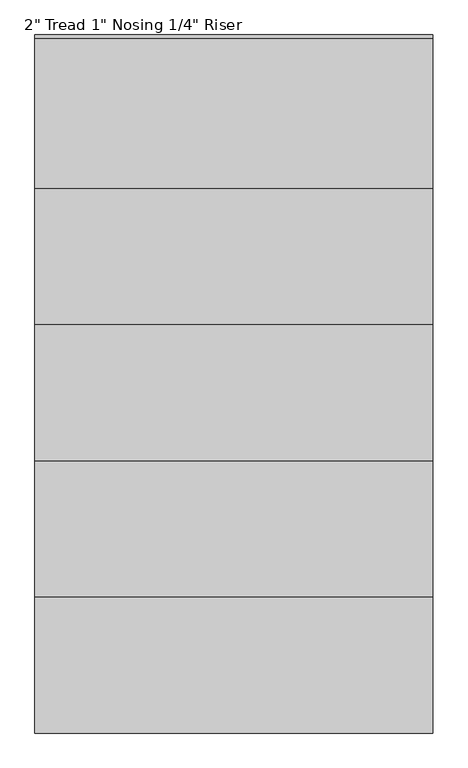
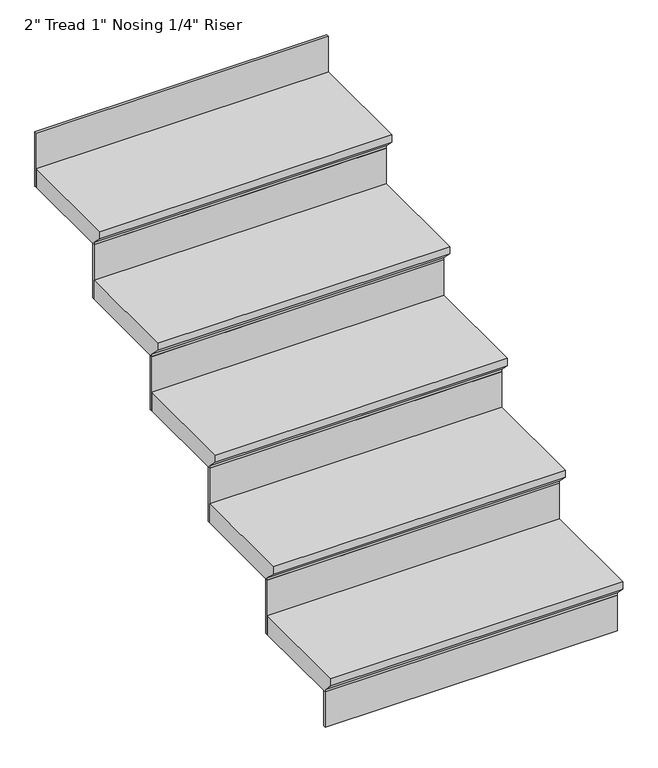
"""IFC4 building model written with IfcOpenShell, lengths in millimetres: stair flight geometry."""

from ifc_helpers import new_model, si_unit, origin, place, context, project, spatial, faceted_brep, source, transform, mapped, element, save


def stair_flight_5ae95f2f(model_context):
    return source(origin(), model_context, "Body", "Brep", [
        faceted_brep([(-5330.5155596, 4813.6076853, 3632.2), (-5330.5155596, 4813.6076853, 3651.25), (-6072.1955596, 4813.6076853, 3651.25), (-6072.1955596, 4813.6076853, 3632.2), (-5330.5155596, 4839.0076853, 3606.8), (-6072.1955596, 4839.0076853, 3606.8), (-5330.5155596, 5093.0076853, 3651.25), (-6072.1955596, 5093.0076853, 3651.25), (-6072.1955596, 4839.0076853, 3600.45), (-6072.1955596, 5093.0076853, 3600.45), (-5330.5155596, 5093.0076853, 3600.45), (-5330.5155596, 4839.0076853, 3600.45)], [[[0, 1, 2, 3]], [[4, 0, 3, 5]], [[2, 1, 6, 7]], [[8, 9, 10, 11]], [[2, 7, 9, 8, 5, 3]], [[8, 11, 4, 5]], [[6, 1, 0, 4, 11, 10]], [[7, 6, 10, 9]]]),
        faceted_brep([(-5330.5155596, 4839.0076853, 3600.45), (-5330.5155596, 4839.0076853, 3505.2), (-5330.5155596, 4845.3576853, 3505.2), (-5330.5155596, 4845.3576853, 3600.45), (-6072.1955596, 4839.0076853, 3600.45), (-6072.1955596, 4845.3576853, 3600.45), (-6072.1955596, 4845.3576853, 3505.2), (-6072.1955596, 4839.0076853, 3505.2)], [[[0, 1, 2, 3]], [[4, 5, 6, 7]], [[1, 0, 4, 7]], [[2, 1, 7, 6]], [[3, 2, 6, 5]], [[0, 3, 5, 4]]]),
        faceted_brep([(-5330.5155596, 5093.0076853, 3746.5), (-5330.5155596, 5093.0076853, 3600.45), (-5330.5155596, 5099.3576853, 3600.45), (-5330.5155596, 5099.3576853, 3746.5), (-6072.1955596, 5093.0076853, 3746.5), (-6072.1955596, 5099.3576853, 3746.5), (-6072.1955596, 5099.3576853, 3600.45), (-6072.1955596, 5093.0076853, 3600.45)], [[[0, 1, 2, 3]], [[4, 5, 6, 7]], [[1, 0, 4, 7]], [[2, 1, 7, 6]], [[3, 2, 6, 5]], [[0, 3, 5, 4]]]),
        faceted_brep([(-6072.1955596, 5067.6076853, 3797.3), (-5330.5155596, 5067.6076853, 3797.3), (-5330.5155596, 5347.0076853, 3797.3), (-6072.1955596, 5347.0076853, 3797.3), (-6072.1955596, 5093.0076853, 3746.5), (-6072.1955596, 5347.0076853, 3746.5), (-5330.5155596, 5347.0076853, 3746.5), (-5330.5155596, 5093.0076853, 3746.5), (-6072.1955596, 5093.0076853, 3752.85), (-6072.1955596, 5067.6076853, 3778.25), (-5330.5155596, 5093.0076853, 3752.85), (-5330.5155596, 5067.6076853, 3778.25)], [[[0, 1, 2, 3]], [[4, 5, 6, 7]], [[0, 3, 5, 4, 8, 9]], [[4, 7, 10, 8]], [[2, 1, 11, 10, 7, 6]], [[3, 2, 6, 5]], [[11, 1, 0, 9]], [[10, 11, 9, 8]]]),
        faceted_brep([(-5330.5155596, 5347.0076853, 3892.55), (-5330.5155596, 5347.0076853, 3746.5), (-5330.5155596, 5353.3576853, 3746.5), (-5330.5155596, 5353.3576853, 3892.55), (-6072.1955596, 5347.0076853, 3892.55), (-6072.1955596, 5353.3576853, 3892.55), (-6072.1955596, 5353.3576853, 3746.5), (-6072.1955596, 5347.0076853, 3746.5)], [[[0, 1, 2, 3]], [[4, 5, 6, 7]], [[1, 0, 4, 7]], [[2, 1, 7, 6]], [[3, 2, 6, 5]], [[0, 3, 5, 4]]]),
        faceted_brep([(-6072.1955596, 5321.6076853, 3943.35), (-5330.5155596, 5321.6076853, 3943.35), (-5330.5155596, 5601.0076853, 3943.35), (-6072.1955596, 5601.0076853, 3943.35), (-6072.1955596, 5347.0076853, 3892.55), (-6072.1955596, 5601.0076853, 3892.55), (-5330.5155596, 5601.0076853, 3892.55), (-5330.5155596, 5347.0076853, 3892.55), (-6072.1955596, 5347.0076853, 3898.9), (-6072.1955596, 5321.6076853, 3924.3), (-5330.5155596, 5347.0076853, 3898.9), (-5330.5155596, 5321.6076853, 3924.3)], [[[0, 1, 2, 3]], [[4, 5, 6, 7]], [[0, 3, 5, 4, 8, 9]], [[4, 7, 10, 8]], [[2, 1, 11, 10, 7, 6]], [[3, 2, 6, 5]], [[11, 1, 0, 9]], [[10, 11, 9, 8]]]),
        faceted_brep([(-5330.5155596, 5601.0076853, 4038.6), (-5330.5155596, 5601.0076853, 3892.55), (-5330.5155596, 5607.3576853, 3892.55), (-5330.5155596, 5607.3576853, 4038.6), (-6072.1955596, 5601.0076853, 4038.6), (-6072.1955596, 5607.3576853, 4038.6), (-6072.1955596, 5607.3576853, 3892.55), (-6072.1955596, 5601.0076853, 3892.55)], [[[0, 1, 2, 3]], [[4, 5, 6, 7]], [[1, 0, 4, 7]], [[2, 1, 7, 6]], [[3, 2, 6, 5]], [[0, 3, 5, 4]]]),
        faceted_brep([(-6072.1955596, 5575.6076853, 4089.4), (-5330.5155596, 5575.6076853, 4089.4), (-5330.5155596, 5855.0076853, 4089.4), (-6072.1955596, 5855.0076853, 4089.4), (-6072.1955596, 5601.0076853, 4038.6), (-6072.1955596, 5855.0076853, 4038.6), (-5330.5155596, 5855.0076853, 4038.6), (-5330.5155596, 5601.0076853, 4038.6), (-6072.1955596, 5601.0076853, 4044.95), (-6072.1955596, 5575.6076853, 4070.35), (-5330.5155596, 5601.0076853, 4044.95), (-5330.5155596, 5575.6076853, 4070.35)], [[[0, 1, 2, 3]], [[4, 5, 6, 7]], [[0, 3, 5, 4, 8, 9]], [[4, 7, 10, 8]], [[2, 1, 11, 10, 7, 6]], [[3, 2, 6, 5]], [[11, 1, 0, 9]], [[10, 11, 9, 8]]]),
        faceted_brep([(-5330.5155596, 6109.0076853, 4330.7), (-5330.5155596, 6109.0076853, 4184.65), (-5330.5155596, 6115.3576853, 4184.65), (-5330.5155596, 6115.3576853, 4330.7), (-6072.1955596, 6109.0076853, 4330.7), (-6072.1955596, 6115.3576853, 4330.7), (-6072.1955596, 6115.3576853, 4184.65), (-6072.1955596, 6109.0076853, 4184.65)], [[[0, 1, 2, 3]], [[4, 5, 6, 7]], [[1, 0, 4, 7]], [[2, 1, 7, 6]], [[3, 2, 6, 5]], [[0, 3, 5, 4]]]),
        faceted_brep([(-5330.5155596, 5855.0076853, 4184.65), (-5330.5155596, 5855.0076853, 4038.6), (-5330.5155596, 5861.3576853, 4038.6), (-5330.5155596, 5861.3576853, 4184.65), (-6072.1955596, 5855.0076853, 4184.65), (-6072.1955596, 5861.3576853, 4184.65), (-6072.1955596, 5861.3576853, 4038.6), (-6072.1955596, 5855.0076853, 4038.6)], [[[0, 1, 2, 3]], [[4, 5, 6, 7]], [[1, 0, 4, 7]], [[2, 1, 7, 6]], [[3, 2, 6, 5]], [[0, 3, 5, 4]]]),
        faceted_brep([(-6072.1955596, 5829.6076853, 4235.45), (-5330.5155596, 5829.6076853, 4235.45), (-5330.5155596, 6083.6076853, 4235.45), (-5330.5155596, 6109.0076853, 4235.45), (-6072.1955596, 6109.0076853, 4235.45), (-6072.1955596, 5855.0076853, 4184.65), (-6072.1955596, 6109.0076853, 4184.65), (-5330.5155596, 6109.0076853, 4184.65), (-5330.5155596, 6083.6076853, 4184.65), (-5330.5155596, 5855.0076853, 4184.65), (-6072.1955596, 5855.0076853, 4191.0), (-6072.1955596, 5829.6076853, 4216.4), (-5330.5155596, 5855.0076853, 4191.0), (-5330.5155596, 5829.6076853, 4216.4)], [[[0, 1, 2, 3, 4]], [[5, 6, 7, 8, 9]], [[0, 4, 6, 5, 10, 11]], [[5, 9, 12, 10]], [[2, 1, 13, 12, 9, 8]], [[3, 2, 8, 7]], [[4, 3, 7, 6]], [[13, 1, 0, 11]], [[12, 13, 11, 10]]]),
    ])


if __name__ == "__main__":
    model = new_model("IFC4")
    model_context = context("Model", 3, world=origin())
    ifc_project = project(units=[si_unit("LENGTHUNIT", "METRE", prefix="MILLI")], contexts=[model_context])
    site = spatial("IfcSite", under=ifc_project)
    building = spatial("IfcBuilding", under=site)
    placement = place(None, origin())
    stair_flight_shape = stair_flight_5ae95f2f(model_context)
    element("IfcStairFlight", 1, ObjectType="2\" Tread 1\" Nosing 1/4\" Riser", at=placement, inside=building, context=model_context, shape_type="MappedRepresentation", body=[
        mapped(stair_flight_shape, transform((0.0, 0.0, 0.0), x_axis=(1.0, 0.0, 0.0), y_axis=(0.0, 1.0, 0.0), z_axis=(0.0, 0.0, 1.0))),
    ])
    save(model, "model.ifc")
